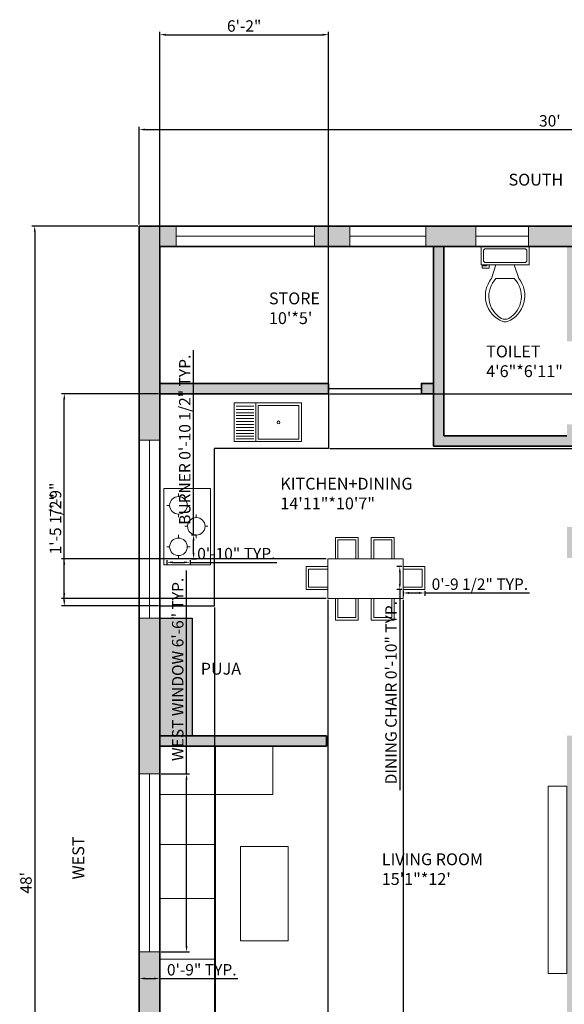
# Model space of a CAD drawing. Units: inches. Extents: x 2066 to 2563, y 1438 to 2142.
# Tile 2 of 3: x 2066 to 2304, y 1710 to 2142. Entities that reach past the tile are written whole.
import ezdxf

# ---------------------------------------------------------------- set-up
doc = ezdxf.new("R2010")
doc.units = ezdxf.units.IN
for name, color, linetype, lineweight in [('A-ANNO-DIMS', 2, 'Continuous', 18), ('A-ANNO-TEXT', 10, 'Continuous', 18), ('A-AREA-IDEN', 10, 'Continuous', 18), ('A-DOOR', 4, 'Continuous', 25), ('A-EQPM', 52, 'Continuous', 18), ('A-FLOR-CASE', 191, 'Continuous', 25), ('A-FLOR-CASE-PATT', 9, 'Continuous', 13), ('A-FLOR-FIXT', 8, 'Continuous', 18), ('A-WALL-PATT', 140, 'Continuous', 13), ('FUR', 191, 'Continuous', 18), ('KIT', 52, 'Continuous', 25), ('WALL', 7, 'Continuous', 35), ('WIND', 210, 'Continuous', 18)]:
    doc.layers.add(name, color=color, linetype=linetype, lineweight=lineweight)
doc.styles.get("Standard").update_dxf_attribs({"font": 'arial.ttf'})
doc.dimstyles.new('ISO-25', dxfattribs={"dimtxt": 5, "dimasz": 2.5, "dimexe": 1.25, "dimexo": 0.625, "dimtad": 1, "dimdec": 0, "dimlunit": 4, "dimtxsty": 'Standard', "dimcen": 2.5, "dimadec": 0, "dimazin": 0, "dimtfac": 1, "dimtdec": 0, "dimtmove": 0, "dimatfit": 3, "dimfxl": 1, "dimarcsym": 0})

# ---------------------------------------------------------------- blocks, each defined once
blk = doc.blocks.new('*U3')
for p, q in [((9.5, -6), (9.5, -2)), ((-10, -8.5), (-8, -8.5)), ((-10, -9.5), (-10, -8.5)), ((-8, -8.5), (-8, -8)), ((-7, -8), (-7, -9.5)), ((-4, -8), (-6, -14)), ((4, -8), (6, -14)), ((-7, -9.5), (-10, -9.5)), ((4, -14), (-4, -14))]:
    blk.add_line(p, q)
blk.add_lwpolyline([(10.5, -8), (10.5, 0), (-10.5, 0), (-10.5, -8)], close=True)
for points in [[(-9.5, -2), (-9.5, -6)], [(8.5, -1), (-8.5, -1)], [(-8.5, -7), (8.5, -7)]]:
    blk.add_lwpolyline(points)
for centre, radius, start, end in [((-8.62, -1.88), 0.884, 81.8699, 188.1301), ((8.62, -1.88), 0.884, 351.8699, 98.1301), ((-8.62, -6.12), 0.884, 171.8699, 278.1301), ((8.62, -6.12), 0.884, 261.8699, 8.1301), ((3.52, -21.58), 12.17, 141.4691, 247.9714), ((4.2, -21.82), 11.33, 136.3677, 238.9468), ((-3.52, -21.58), 12.17, 292.0284, 38.5307), ((-4.2, -21.82), 11.33, 301.053, 43.6321), ((0, -27.88), 4, 245.7318, 294.2682), ((0, -29), 4, 254.8605, 285.1395)]:
    blk.add_arc(centre, radius, start, end)
blk = doc.blocks.new('*D8')
at = {"layer": 'A-ANNO-DIMS', "color": 0, "lineweight": -2, "transparency": 16777216}
for p, q in [((2118.07, 2051.67), (2118.07, 2094.59)), ((2478.07, 2051.67), (2478.07, 2094.59)), ((2120.57, 2093.34), (2475.57, 2093.34))]:
    blk.add_line(p, q, dxfattribs=at)
at = {"layer": 'A-ANNO-DIMS', "color": 0, "lineweight": 100, "transparency": 16777216}
for points in [[(2120.57, 2093.76), (2120.57, 2092.93), (2118.07, 2093.34)], [(2475.57, 2093.76), (2475.57, 2092.93), (2478.07, 2093.34)]]:
    blk.add_solid(points, dxfattribs=at)
at = {"layer": 'Defpoints', "color": 0, "lineweight": 100, "transparency": 16777216}
for p in [(2478.07, 2093.34), (2118.07, 2051.04), (2478.07, 2051.04)]:
    blk.add_point(p, dxfattribs=at)
at = {"layer": 'A-ANNO-DIMS', "color": 0, "transparency": 16777216, "insert": (2298.07, 2096.52), "char_height": 5, "attachment_point": 5}
blk.add_mtext("30'", dxfattribs=at)
blk = doc.blocks.new('*D9')
at = {"layer": 'A-ANNO-DIMS', "color": 0, "lineweight": -2, "transparency": 16777216}
for p, q in [((2117.45, 2051.04), (2070.96, 2051.04)), ((2072.21, 2048.54), (2072.21, 1477.54)), ((2117.45, 1475.04), (2070.96, 1475.04))]:
    blk.add_line(p, q, dxfattribs=at)
at = {"layer": 'A-ANNO-DIMS', "color": 0, "lineweight": 100, "transparency": 16777216}
for points in [[(2071.79, 2048.54), (2072.63, 2048.54), (2072.21, 2051.04)], [(2071.79, 1477.54), (2072.63, 1477.54), (2072.21, 1475.04)]]:
    blk.add_solid(points, dxfattribs=at)
at = {"layer": 'Defpoints', "color": 0, "lineweight": 100, "transparency": 16777216}
for p in [(2118.07, 2051.04), (2072.21, 1475.04), (2118.07, 1475.04)]:
    blk.add_point(p, dxfattribs=at)
at = {"layer": 'A-ANNO-DIMS', "color": 0, "transparency": 16777216, "insert": (2069.03, 1763.04), "char_height": 5, "attachment_point": 5, "rotation": 90}
blk.add_mtext("48'", dxfattribs=at)
blk = doc.blocks.new('CHAIR-DINING')
for p, q in [((0, 0), (0, 9.41)), ((0, 9.41), (10.07, 9.41)), ((10.07, 9.41), (10.07, 0))]:
    blk.add_line(p, q)
blk.add_lwpolyline([(1.13, 0), (9, 0), (9, 8.36), (1.13, 8.36)], close=True)
blk = doc.blocks.new('COOKTOP-BURNER')
for p, q in [((5.08, 9.08), (5.08, 10.45)), ((0, 5.22), (1.22, 5.22)), ((8.93, 5.22), (10.15, 5.22)), ((5.08, 0), (5.08, 1.37))]:
    blk.add_line(p, q)
blk.add_circle((5.08, 5.22), 3.85)
blk = doc.blocks.new('WIN-78IN')
blk.add_line((4.5, 78.03), (4.5, 0))
blk.add_lwpolyline([(0, 0), (9, 0), (9, 78.03), (0, 78.03)], close=True)
blk = doc.blocks.new('*D16')
at = {"layer": 'A-ANNO-DIMS', "color": 0, "lineweight": -2, "transparency": 16777216}
for p, q in [((2233.18, 1901.72), (2231.04, 1901.72)), ((2232.29, 1899.22), (2232.29, 1894.15)), ((2233.18, 1891.65), (2231.04, 1891.65)), ((2232.29, 1891.65), (2232.29, 1803.73))]:
    blk.add_line(p, q, dxfattribs=at)
at = {"layer": 'A-ANNO-DIMS', "color": 0, "lineweight": 100, "transparency": 16777216}
for points in [[(2231.88, 1899.22), (2232.71, 1899.22), (2232.29, 1901.72)], [(2231.88, 1894.15), (2232.71, 1894.15), (2232.29, 1891.65)]]:
    blk.add_solid(points, dxfattribs=at)
at = {"layer": 'Defpoints', "color": 0, "lineweight": 100, "transparency": 16777216}
for p in [(2233.8, 1901.72), (2232.29, 1891.65), (2233.8, 1891.65)]:
    blk.add_point(p, dxfattribs=at)
at = {"layer": 'A-ANNO-DIMS', "color": 0, "transparency": 16777216, "insert": (2229.08, 1846.44), "char_height": 5, "attachment_point": 5, "rotation": 90}
blk.add_mtext('DINING CHAIR 0\'-10" TYP.', dxfattribs=at)
blk = doc.blocks.new('*D17')
at = {"layer": 'A-ANNO-DIMS', "color": 0, "lineweight": -2, "transparency": 16777216}
for p, q in [((2233.8, 1891.03), (2233.8, 1888.89)), ((2236.3, 1890.14), (2240.72, 1890.14)), ((2243.22, 1891.03), (2243.22, 1888.89)), ((2243.22, 1890.14), (2289.09, 1890.14))]:
    blk.add_line(p, q, dxfattribs=at)
at = {"layer": 'A-ANNO-DIMS', "color": 0, "lineweight": 100, "transparency": 16777216}
for points in [[(2236.3, 1890.56), (2236.3, 1889.72), (2233.8, 1890.14)], [(2240.72, 1890.56), (2240.72, 1889.72), (2243.22, 1890.14)]]:
    blk.add_solid(points, dxfattribs=at)
at = {"layer": 'Defpoints', "color": 0, "lineweight": 100, "transparency": 16777216}
for p in [(2233.8, 1891.65), (2243.22, 1891.65), (2243.22, 1890.14)]:
    blk.add_point(p, dxfattribs=at)
at = {"layer": 'A-ANNO-DIMS', "color": 0, "transparency": 16777216, "insert": (2267.4, 1893.35), "char_height": 5, "attachment_point": 5}
blk.add_mtext('0\'-9 1/2" TYP.', dxfattribs=at)
blk = doc.blocks.new('*D20')
at = {"layer": 'A-ANNO-DIMS', "color": 0, "lineweight": -2, "transparency": 16777216}
for p, q in [((2141.87, 1915.6), (2141.87, 1996.57)), ((2140.93, 1915.6), (2143.12, 1915.6)), ((2141.87, 1907.65), (2141.87, 1913.1)), ((2140.93, 1905.15), (2143.12, 1905.15))]:
    blk.add_line(p, q, dxfattribs=at)
at = {"layer": 'A-ANNO-DIMS', "color": 0, "lineweight": 100, "transparency": 16777216}
for points in [[(2141.45, 1913.1), (2142.29, 1913.1), (2141.87, 1915.6)], [(2141.45, 1907.65), (2142.29, 1907.65), (2141.87, 1905.15)]]:
    blk.add_solid(points, dxfattribs=at)
at = {"layer": 'Defpoints', "color": 0, "lineweight": 100, "transparency": 16777216}
for p in [(2140.3, 1915.6), (2141.87, 1915.6), (2140.3, 1905.15)]:
    blk.add_point(p, dxfattribs=at)
at = {"layer": 'A-ANNO-DIMS', "color": 0, "transparency": 16777216, "insert": (2138.66, 1957.34), "char_height": 5, "attachment_point": 5, "rotation": 90}
blk.add_mtext('BURNER 0\'-10 1/2" TYP.', dxfattribs=at)
blk = doc.blocks.new('*D21')
at = {"layer": 'A-ANNO-DIMS', "color": 0, "lineweight": -2, "transparency": 16777216}
for p, q in [((2130.15, 1904.52), (2130.15, 1902.33)), ((2140.3, 1904.52), (2140.3, 1902.33)), ((2132.65, 1903.58), (2137.8, 1903.58)), ((2140.3, 1903.58), (2178.41, 1903.58))]:
    blk.add_line(p, q, dxfattribs=at)
at = {"layer": 'A-ANNO-DIMS', "color": 0, "lineweight": 100, "transparency": 16777216}
for points in [[(2132.65, 1904), (2132.65, 1903.17), (2130.15, 1903.58)], [(2137.8, 1904), (2137.8, 1903.17), (2140.3, 1903.58)]]:
    blk.add_solid(points, dxfattribs=at)
at = {"layer": 'Defpoints', "color": 0, "lineweight": 100, "transparency": 16777216}
for p in [(2130.15, 1905.15), (2140.3, 1905.15), (2140.3, 1903.58)]:
    blk.add_point(p, dxfattribs=at)
at = {"layer": 'A-ANNO-DIMS', "color": 0, "transparency": 16777216, "insert": (2160.61, 1906.76), "char_height": 5, "attachment_point": 5}
blk.add_mtext('0\'-10" TYP.', dxfattribs=at)
blk = doc.blocks.new('*D24')
at = {"layer": 'A-ANNO-DIMS', "color": 0, "lineweight": -2, "transparency": 16777216}
for p, q in [((2138.78, 1810.83), (2138.78, 1899.97)), ((2127.7, 1810.83), (2140.03, 1810.83)), ((2138.78, 1735.3), (2138.78, 1808.33)), ((2127.7, 1732.8), (2140.03, 1732.8))]:
    blk.add_line(p, q, dxfattribs=at)
at = {"layer": 'A-ANNO-DIMS', "color": 0, "lineweight": 100, "transparency": 16777216}
for points in [[(2138.36, 1808.33), (2139.19, 1808.33), (2138.78, 1810.83)], [(2138.36, 1735.3), (2139.19, 1735.3), (2138.78, 1732.8)]]:
    blk.add_solid(points, dxfattribs=at)
at = {"layer": 'Defpoints', "color": 0, "lineweight": 100, "transparency": 16777216}
for p in [(2127.07, 1810.83), (2138.78, 1810.83), (2127.07, 1732.8)]:
    blk.add_point(p, dxfattribs=at)
at = {"layer": 'A-ANNO-DIMS', "color": 0, "transparency": 16777216, "insert": (2135.57, 1856.65), "char_height": 5, "attachment_point": 5, "rotation": 90}
blk.add_mtext('WEST WINDOW 6\'-6" TYP.', dxfattribs=at)
blk = doc.blocks.new('*D25')
at = {"layer": 'A-ANNO-DIMS', "color": 0, "lineweight": -2, "transparency": 16777216}
for p, q in [((2118.07, 1732.17), (2118.07, 1719.84)), ((2127.07, 1732.17), (2127.07, 1719.84)), ((2120.57, 1721.09), (2124.57, 1721.09)), ((2127.07, 1721.09), (2161.3, 1721.09))]:
    blk.add_line(p, q, dxfattribs=at)
at = {"layer": 'A-ANNO-DIMS', "color": 0, "lineweight": 100, "transparency": 16777216}
for points in [[(2120.57, 1721.51), (2120.57, 1720.68), (2118.07, 1721.09)], [(2124.57, 1721.51), (2124.57, 1720.68), (2127.07, 1721.09)]]:
    blk.add_solid(points, dxfattribs=at)
at = {"layer": 'Defpoints', "color": 0, "lineweight": 100, "transparency": 16777216}
for p in [(2118.07, 1732.8), (2127.07, 1732.8), (2127.07, 1721.09)]:
    blk.add_point(p, dxfattribs=at)
at = {"layer": 'A-ANNO-DIMS', "color": 0, "transparency": 16777216, "insert": (2145.44, 1724.27), "char_height": 5, "attachment_point": 5}
blk.add_mtext('0\'-9" TYP.', dxfattribs=at)
blk = doc.blocks.new('*D30')
at = {"layer": 'A-ANNO-DIMS', "color": 0, "lineweight": -2, "transparency": 16777216}
for p, q in [((2127.07, 1883.82), (2127.07, 1440.89)), ((2151.07, 1883.82), (2151.07, 1440.89)), ((2129.57, 1442.14), (2148.57, 1442.14))]:
    blk.add_line(p, q, dxfattribs=at)
at = {"layer": 'A-ANNO-DIMS', "color": 0, "lineweight": 100, "transparency": 16777216}
for points in [[(2129.57, 1442.56), (2129.57, 1441.73), (2127.07, 1442.14)], [(2148.57, 1442.56), (2148.57, 1441.73), (2151.07, 1442.14)]]:
    blk.add_solid(points, dxfattribs=at)
at = {"layer": 'Defpoints', "color": 0, "lineweight": 100, "transparency": 16777216}
for p in [(2127.07, 1884.45), (2151.07, 1884.45), (2151.07, 1442.14)]:
    blk.add_point(p, dxfattribs=at)
at = {"layer": 'A-ANNO-DIMS', "color": 0, "transparency": 16777216, "insert": (2139.07, 1445.32), "char_height": 5, "attachment_point": 5}
blk.add_mtext('2\'-0"', dxfattribs=at)
blk = doc.blocks.new('*D31')
at = {"layer": 'A-ANNO-DIMS', "color": 0, "lineweight": -2, "transparency": 16777216}
for p, q in [((2126.45, 1977.54), (2083.92, 1977.54)), ((2085.17, 1886.95), (2085.17, 1975.04)), ((2126.45, 1884.45), (2083.92, 1884.45))]:
    blk.add_line(p, q, dxfattribs=at)
at = {"layer": 'A-ANNO-DIMS', "color": 0, "lineweight": 100, "transparency": 16777216}
for points in [[(2084.76, 1975.04), (2085.59, 1975.04), (2085.17, 1977.54)], [(2084.76, 1886.95), (2085.59, 1886.95), (2085.17, 1884.45)]]:
    blk.add_solid(points, dxfattribs=at)
at = {"layer": 'Defpoints', "color": 0, "lineweight": 100, "transparency": 16777216}
for p in [(2085.17, 1977.54), (2127.07, 1977.54), (2127.07, 1884.45)]:
    blk.add_point(p, dxfattribs=at)
at = {"layer": 'A-ANNO-DIMS', "color": 0, "transparency": 16777216, "insert": (2082, 1931), "char_height": 5, "attachment_point": 5, "rotation": 90}
blk.add_mtext('7\'-9"', dxfattribs=at)
blk = doc.blocks.new('*D32')
at = {"layer": 'A-ANNO-DIMS', "color": 0, "lineweight": -2, "transparency": 16777216}
for p, q in [((2127.07, 1978.17), (2127.07, 2136.19)), ((2129.57, 2134.94), (2198.51, 2134.94)), ((2201.01, 1978.17), (2201.01, 2136.19))]:
    blk.add_line(p, q, dxfattribs=at)
at = {"layer": 'A-ANNO-DIMS', "color": 0, "lineweight": 100, "transparency": 16777216}
for points in [[(2129.57, 2135.36), (2129.57, 2134.53), (2127.07, 2134.94)], [(2198.51, 2135.36), (2198.51, 2134.53), (2201.01, 2134.94)]]:
    blk.add_solid(points, dxfattribs=at)
at = {"layer": 'Defpoints', "color": 0, "lineweight": 100, "transparency": 16777216}
for p in [(2201.01, 2134.94), (2127.07, 1977.54), (2201.01, 1977.54)]:
    blk.add_point(p, dxfattribs=at)
at = {"layer": 'A-ANNO-DIMS', "color": 0, "transparency": 16777216, "insert": (2164.04, 2138.12), "char_height": 5, "attachment_point": 5}
blk.add_mtext('6\'-2"', dxfattribs=at)
blk = doc.blocks.new('*D33')
at = {"layer": 'A-ANNO-DIMS', "color": 0, "lineweight": -2, "transparency": 16777216}
for p, q in [((2201.63, 1977.54), (2563.22, 1977.54)), ((2561.97, 1975.04), (2561.97, 1956.04)), ((2201.63, 1953.54), (2563.22, 1953.54))]:
    blk.add_line(p, q, dxfattribs=at)
at = {"layer": 'A-ANNO-DIMS', "color": 0, "lineweight": 100, "transparency": 16777216}
for points in [[(2561.56, 1975.04), (2562.39, 1975.04), (2561.97, 1977.54)], [(2561.56, 1956.04), (2562.39, 1956.04), (2561.97, 1953.54)]]:
    blk.add_solid(points, dxfattribs=at)
at = {"layer": 'Defpoints', "color": 0, "lineweight": 100, "transparency": 16777216}
for p in [(2201.01, 1977.54), (2201.01, 1953.54), (2561.97, 1953.54)]:
    blk.add_point(p, dxfattribs=at)
at = {"layer": 'A-ANNO-DIMS', "color": 0, "transparency": 16777216, "insert": (2558.8, 1965.54), "char_height": 5, "attachment_point": 5, "rotation": 90}
blk.add_mtext('2\'-0"', dxfattribs=at)
blk = doc.blocks.new('*D34')
at = {"layer": 'A-ANNO-DIMS', "color": 0, "lineweight": -2, "transparency": 16777216}
for p, q in [((2200.67, 1887.07), (2200.67, 1440.89)), ((2233.8, 1887.07), (2233.8, 1440.89)), ((2203.17, 1442.14), (2231.3, 1442.14))]:
    blk.add_line(p, q, dxfattribs=at)
at = {"layer": 'A-ANNO-DIMS', "color": 0, "lineweight": 100, "transparency": 16777216}
for points in [[(2203.17, 1442.56), (2203.17, 1441.73), (2200.67, 1442.14)], [(2231.3, 1442.56), (2231.3, 1441.73), (2233.8, 1442.14)]]:
    blk.add_solid(points, dxfattribs=at)
at = {"layer": 'Defpoints', "color": 0, "lineweight": 100, "transparency": 16777216}
for p in [(2200.67, 1887.69), (2233.8, 1887.69), (2233.8, 1442.14)]:
    blk.add_point(p, dxfattribs=at)
at = {"layer": 'A-ANNO-DIMS', "color": 0, "transparency": 16777216, "insert": (2217.24, 1445.32), "char_height": 5, "attachment_point": 5}
blk.add_mtext('2\'-9"', dxfattribs=at)
blk = doc.blocks.new('*D35')
at = {"layer": 'A-ANNO-DIMS', "color": 0, "lineweight": -2, "transparency": 16777216}
for p, q in [((2085.17, 1905.12), (2085.17, 1933.35)), ((2200.04, 1905.12), (2083.92, 1905.12)), ((2085.17, 1890.19), (2085.17, 1902.62)), ((2200.04, 1887.69), (2083.92, 1887.69))]:
    blk.add_line(p, q, dxfattribs=at)
at = {"layer": 'A-ANNO-DIMS', "color": 0, "lineweight": 100, "transparency": 16777216}
for points in [[(2084.76, 1902.62), (2085.59, 1902.62), (2085.17, 1905.12)], [(2084.76, 1890.19), (2085.59, 1890.19), (2085.17, 1887.69)]]:
    blk.add_solid(points, dxfattribs=at)
at = {"layer": 'Defpoints', "color": 0, "lineweight": 100, "transparency": 16777216}
for p in [(2085.17, 1905.12), (2200.67, 1905.12), (2200.67, 1887.69)]:
    blk.add_point(p, dxfattribs=at)
at = {"layer": 'A-ANNO-DIMS', "color": 0, "transparency": 16777216, "insert": (2081.96, 1920.48), "char_height": 5, "attachment_point": 5, "rotation": 90}
blk.add_mtext('1\'-5 1/2"', dxfattribs=at)

msp = doc.modelspace()

# ---------------------------------------------------------------- hatches: boundary and pattern name
at = {"layer": 'A-FLOR-CASE-PATT'}
h = msp.add_hatch(color=256, dxfattribs=at)
h.dxf.hatch_style = 1
h.paths.add_polyline_path([(2141.31, 1879.08), (2127.07, 1879.08), (2127.07, 1827.54), (2141.31, 1827.54)])
at = {"layer": 'A-WALL-PATT'}
h = msp.add_hatch(color=256, dxfattribs=at)
h.dxf.hatch_style = 1
h.paths.add_polyline_path([(2210.43, 2051.04), (2194.82, 2051.04), (2194.82, 2042.04), (2210.43, 2042.04)])
h.paths.add_polyline_path([(2265.69, 2051.04), (2243.73, 2051.04), (2243.73, 2042.04), (2265.69, 2042.04)])
h.paths.add_polyline_path([(2478.07, 2051.04), (2288.73, 2051.04), (2288.73, 2042.04), (2288.96, 2042.04), (2469.07, 2042.04), (2469.07, 2021.26), (2478.07, 2021.26)])
h.paths.add_polyline_path([(2127.07, 2042.04), (2134.17, 2042.04), (2134.17, 2051.04), (2118.07, 2051.04), (2118.07, 1957.11), (2127.07, 1957.11), (2127.07, 1977.54)])
h.paths.add_polyline_path([(2201.01, 1982.04), (2127.07, 1982.04), (2127.07, 1977.54), (2201.01, 1977.54)])
h.paths.add_polyline_path([(2247.07, 1982.04), (2241.78, 1982.04), (2241.78, 1977.54), (2247.07, 1977.54)])
h.paths.add_polyline_path([(2251.57, 2042.04), (2247.07, 2042.04), (2247.07, 1954.54), (2310.07, 1954.54), (2310.07, 1964.11), (2305.57, 1964.11), (2305.57, 1959.04), (2251.57, 1959.04)])
h.paths.add_polyline_path([(2310.07, 2042.04), (2305.57, 2042.04), (2305.57, 2000.54), (2310.07, 2000.54)], flags=17)
h.paths.add_polyline_path([(2478.07, 1938.37), (2469.07, 1938.37), (2469.07, 1846.24), (2478.07, 1846.24)])
h.paths.add_polyline_path([(2469.07, 1910.04), (2384.89, 1910.04), (2370.05, 1910.04), (2318.28, 1910.04), (2310.07, 1910.04), (2310.07, 1919.07), (2305.57, 1919.07), (2305.57, 1910.04), (2305.57, 1905.54), (2310.07, 1905.54), (2318.28, 1905.54), (2370.05, 1905.54), (2469.07, 1905.54)])
h.paths.add_polyline_path([(2469.07, 1868.54), (2408.15, 1868.54), (2408.15, 1858.69), (2412.15, 1858.69), (2412.15, 1864.54), (2469.07, 1864.54)])
h.paths.add_polyline_path([(2469.07, 1827.54), (2359.25, 1827.54), (2359.25, 1823.04), (2469.07, 1823.04)])
h.paths.add_polyline_path([(2314.44, 1827.54), (2310.07, 1827.54), (2305.57, 1827.54), (2305.57, 1743.86), (2305.57, 1723.24), (2305.57, 1679.04), (2305.57, 1674.54), (2322.38, 1674.54), (2380.79, 1674.54), (2397.77, 1674.54), (2415.18, 1674.54), (2415.18, 1679.04), (2310.07, 1679.04), (2310.07, 1823.04), (2314.44, 1823.04)])
h.paths.add_polyline_path([(2478.07, 1763.36), (2469.07, 1763.36), (2469.07, 1655.36), (2478.07, 1655.36)])
h.paths.add_polyline_path([(2469.07, 1679.04), (2446.03, 1679.04), (2446.03, 1674.54), (2469.07, 1674.54)])
h.paths.add_polyline_path([(2410.07, 1670.54), (2410.07, 1674.54), (2405.57, 1674.54), (2405.57, 1670.54), (2405.57, 1590.09), (2410.07, 1590.09), (2410.07, 1593.54)])
h.paths.add_polyline_path([(2469.07, 1598.04), (2410.07, 1598.04), (2410.07, 1593.54), (2469.07, 1593.54)])
h.paths.add_polyline_path([(2478.07, 1622.1), (2469.07, 1622.1), (2469.07, 1578.59), (2478.07, 1578.59)])
h.paths.add_polyline_path([(2478.07, 1545.33), (2469.07, 1545.33), (2469.07, 1521.54), (2384.6, 1521.54), (2384.6, 1512.54), (2473.57, 1512.54), (2478.07, 1512.54)])
h.paths.add_polyline_path([(2410.07, 1558.62), (2405.57, 1558.62), (2405.57, 1521.54), (2410.07, 1521.54)])
h.paths.add_polyline_path([(2478.07, 1512.54), (2473.57, 1512.54), (2473.57, 1479.54), (2263.07, 1479.54), (2251.16, 1479.54), (2251.16, 1475.04), (2478.07, 1475.04)])
h.paths.add_polyline_path([(2122.57, 1674.54), (2118.07, 1674.54), (2118.07, 1475.04), (2131.87, 1475.04), (2131.87, 1479.54), (2122.57, 1479.54)])
h.paths.add_polyline_path([(2267.57, 1674.54), (2263.07, 1674.54), (2263.07, 1521.54), (2267.57, 1521.54)])
h.paths.add_polyline_path([(2270.46, 1679.04), (2259.18, 1679.04), (2259.18, 1674.54), (2263.07, 1674.54), (2270.46, 1674.54)])
h.paths.add_polyline_path([(2198.77, 1679.04), (2190.12, 1679.04), (2190.12, 1674.54), (2198.77, 1674.54)])
h.paths.add_polyline_path([(2139.93, 1679.04), (2127.07, 1679.04), (2127.07, 1674.54), (2139.93, 1674.54)])
h.paths.add_polyline_path([(2127.07, 1700.37), (2127.07, 1732.8), (2118.07, 1732.8), (2118.07, 1674.54), (2122.57, 1674.54), (2127.07, 1674.54), (2127.07, 1679.04)])
h.paths.add_polyline_path([(2127.07, 1879.08), (2118.07, 1879.08), (2118.07, 1810.83), (2127.07, 1810.83), (2127.07, 1823.04)])
h.paths.add_polyline_path([(2200.14, 1827.54), (2127.07, 1827.54), (2127.07, 1823.04), (2151.5, 1823.04), (2176.6, 1823.04), (2200.14, 1823.04)])

# ---------------------------------------------------------------- linework, layer by layer
at = {"layer": 'A-DOOR'}
msp.add_line((2201.01, 1979.79), (2241.78, 1979.79), dxfattribs=at)
at = {"layer": 'A-EQPM'}
msp.add_lwpolyline([(2128.79, 1902.53), (2149.34, 1902.53), (2149.34, 1935.94), (2128.79, 1935.94)], close=True, dxfattribs=at)
at = {"layer": 'A-FLOR-CASE'}
msp.add_lwpolyline([(2127.07, 1879.08), (2141.31, 1879.08), (2141.31, 1827.54), (2127.07, 1827.54)], close=True, dxfattribs=at)
at = {"layer": 'A-FLOR-FIXT'}
for p, q in [((2169.21, 1973.45), (2169.21, 1956.59)), ((2160.49, 1972.01), (2168.31, 1972.01)), ((2160.49, 1970.66), (2168.31, 1970.66)), ((2160.49, 1969.2), (2168.31, 1969.2)), ((2160.49, 1967.9), (2168.31, 1967.9)), ((2160.49, 1966.6), (2168.31, 1966.6)), ((2160.49, 1965.4), (2168.31, 1965.4)), ((2160.49, 1964), (2168.31, 1964)), ((2160.49, 1962.74), (2168.31, 1962.74)), ((2160.49, 1961.39), (2168.31, 1961.39)), ((2160.49, 1960.14), (2168.31, 1960.14)), ((2160.49, 1958.89), (2168.31, 1958.89)), ((2160.49, 1957.79), (2168.31, 1957.79))]:
    msp.add_line(p, q, dxfattribs=at)
for points in [[(2159.71, 1973.45), (2189.13, 1973.45), (2189.13, 1956.59), (2159.71, 1956.59)], [(2170.26, 1972.31), (2187.96, 1972.31), (2187.96, 1957.58), (2170.26, 1957.58)]]:
    msp.add_lwpolyline(points, close=True, dxfattribs=at)
msp.add_circle((2179.11, 1964.95), 0.627, dxfattribs=at)
at = {"layer": 'FUR'}
for p, q in [((2127.07, 1779.89), (2151.5, 1779.89)), ((2127.07, 1756.23), (2151.5, 1756.23)), ((2127.07, 1729.54), (2151.5, 1729.54))]:
    msp.add_line(p, q, dxfattribs=at)
for points in [[(2200.67, 1905.12), (2233.8, 1905.12), (2233.8, 1887.69), (2200.67, 1887.69)], [(2176.6, 1823.04), (2127.07, 1823.04), (2127.07, 1801.72), (2176.6, 1801.72)], [(2127.07, 1823.04), (2151.5, 1823.04), (2151.5, 1679.04), (2127.07, 1679.04)], [(2305.57, 1805.39), (2297.27, 1805.39), (2297.27, 1723.24), (2305.57, 1723.24)], [(2162.42, 1737.61), (2183.37, 1737.61), (2183.37, 1779.02), (2162.42, 1779.02)]]:
    msp.add_lwpolyline(points, close=True, dxfattribs=at)
at = {"layer": 'KIT'}
for p, q in [((2201.01, 1977.54), (2201.01, 1953.54)), ((2201.01, 1953.54), (2151, 1953.54)), ((2151.07, 1884.45), (2151.07, 1953.54)), ((2127.07, 1884.45), (2151.07, 1884.45))]:
    msp.add_line(p, q, dxfattribs=at)
at = {"layer": 'WALL'}
for p, q in [((2118.07, 2051.04), (2478.07, 2051.04)), ((2118.07, 1475.04), (2118.07, 2051.04)), ((2127.07, 2042.04), (2469.07, 2042.04)), ((2127.07, 2042.04), (2247.07, 2042.04)), ((2127.07, 1674.54), (2127.07, 2042.04)), ((2247.07, 2042.04), (2247.07, 1982.04)), ((2247.07, 2042.04), (2247.07, 1954.54)), ((2251.57, 2042.04), (2251.57, 1977.54)), ((2251.57, 2042.04), (2251.57, 1959.04)), ((2201.01, 1982.04), (2127.07, 1982.04)), ((2201.01, 1982.04), (2201.01, 1977.54)), ((2247.07, 1982.04), (2241.78, 1982.04)), ((2127.07, 1977.54), (2127.07, 1827.54)), ((2201.01, 1977.54), (2127.07, 1977.54)), ((2247.07, 1977.54), (2241.78, 1977.54)), ((2251.57, 1959.04), (2305.57, 1959.04)), ((2247.07, 1954.54), (2310.07, 1954.54)), ((2127.07, 1827.54), (2200.14, 1827.54)), ((2200.14, 1827.54), (2200.14, 1823.04)), ((2127.07, 1823.04), (2200.14, 1823.04)), ((2127.07, 1823.04), (2127.07, 1679.04))]:
    msp.add_line(p, q, dxfattribs=at)
msp.add_lwpolyline([(2241.78, 1982.04), (2241.78, 1982.04), (2241.78, 1977.54), (2241.78, 1977.54)], close=True, dxfattribs=at)
at = {"layer": 'WIND'}
for p, q in [((2134.17, 2046.54), (2194.82, 2046.54)), ((2210.43, 2046.54), (2243.73, 2046.54)), ((2265.69, 2046.54), (2288.73, 2046.54))]:
    msp.add_line(p, q, dxfattribs=at)
for points in [[(2134.17, 2051.04), (2194.82, 2051.04), (2194.82, 2042.04), (2134.17, 2042.04)], [(2243.73, 2042.04), (2210.43, 2042.04), (2210.43, 2051.04), (2243.73, 2051.04)], [(2265.69, 2042.04), (2288.73, 2042.04), (2288.73, 2051.04), (2265.69, 2051.04)]]:
    msp.add_lwpolyline(points, close=True, dxfattribs=at)

# ---------------------------------------------------------------- block references
at = {"layer": 'A-EQPM'}
for p in [(2130.15, 1923.35), (2137.97, 1914.15), (2130.15, 1905.15)]:
    msp.add_blockref('COOKTOP-BURNER', p, dxfattribs=at)
at = {"layer": 'A-FLOR-FIXT'}
msp.add_blockref('*U3', (2278.46, 2042.04), dxfattribs=at)
at = {"layer": 'FUR'}
for p in [(2204.03, 1905.12), (2219.73, 1905.12)]:
    msp.add_blockref('CHAIR-DINING', p, dxfattribs=at)
at = {"layer": 'FUR', "extrusion": (0, 0, -1), "zscale": -1}
for p, rotation in [((-2200.67, 1901.72), 269.9999999999988), ((-2204.03, 1887.69), 180), ((-2219.73, 1887.69), 180)]:
    msp.add_blockref('CHAIR-DINING', p, dxfattribs=dict(at, rotation=rotation))
at = {"layer": 'FUR', "rotation": 269.9999999999988}
msp.add_blockref('CHAIR-DINING', (2233.8, 1901.72), dxfattribs=at)
at = {"layer": 'WIND'}
for p in [(2118.07, 1879.08), (2118.07, 1732.8)]:
    msp.add_blockref('WIN-78IN', p, dxfattribs=at)

# ---------------------------------------------------------------- texts
at = {"layer": 'A-ANNO-TEXT', "insert": (2279.98, 2073.97), "char_height": 5.193, "attachment_point": 1}
msp.add_mtext_dynamic_manual_height_columns('SOUTH', width=129.7814, gutter_width=25.96, heights=[0], dxfattribs=at)
at = {"layer": 'A-ANNO-TEXT', "insert": (2088.72, 1764.51), "char_height": 5.193, "attachment_point": 1, "rotation": 90}
msp.add_mtext_dynamic_manual_height_columns('WEST', width=129.7814, gutter_width=25.96, heights=[0], dxfattribs=at)
at = {"layer": 'A-AREA-IDEN', "attachment_point": 1}
for s, insert, char_height in [("STORE\\P10'*5'", (2174.91, 2021.91), 5.193), ('TOILET\\P4\'6"*6\'11"', (2270.17, 1998.65), 5.193), ('KITCHEN+DINING\\P14\'11"*10\'7"', (2179.92, 1940.66), 5.1929), ('PUJA', (2145, 1859.52), 5.193), ('LIVING ROOM\\P15\'1"*12\'', (2224.38, 1775.97), 5.1929)]:
    msp.add_mtext_dynamic_manual_height_columns(s, width=129.7814, gutter_width=25.96, heights=[0], dxfattribs=dict(at, insert=insert, char_height=char_height))

# ---------------------------------------------------------------- dimensions: what is measured, and where the dimension line sits
at = {"layer": 'A-ANNO-DIMS'}
for base, p1, p2, override, picture, middle in [((2201.01, 2134.94), (2127.07, 1977.54), (2201.01, 1977.54), {"dimdec": 1, "dimlfac": 1, "dimrnd": 0, "dimzin": 1, "dimdsep": 46, "dimlunit": 4, "dimfrac": 2}, '*D32', (2164.04, 2138.12)), ((2478.07, 2093.34), (2118.07, 2051.04), (2478.07, 2051.04), {"dimclrd": 0, "dimclre": 0, "dimclrt": 0}, '*D8', (2298.07, 2096.52)), ((2233.8, 1442.14), (2200.67, 1887.69), (2233.8, 1887.69), {"dimdec": 1, "dimlfac": 1, "dimrnd": 0, "dimzin": 1, "dimdsep": 46, "dimlunit": 4, "dimfrac": 2}, '*D34', (2217.24, 1445.32)), ((2151.07, 1442.14), (2127.07, 1884.45), (2151.07, 1884.45), {"dimdec": 1, "dimlfac": 1, "dimrnd": 0, "dimzin": 1, "dimdsep": 46, "dimlunit": 4, "dimfrac": 2}, '*D30', (2139.07, 1445.32))]:
    dim = msp.add_linear_dim(base=base, p1=p1, p2=p2, dimstyle='ISO-25', override=override, dxfattribs=at)
    dim.commit()
    dim.dimension.update_dxf_attribs({"geometry": picture, "text_midpoint": middle})
for base, p1, p2, override, picture, middle in [((2072.21, 1475.04), (2118.07, 2051.04), (2118.07, 1475.04), {"dimclrd": 0, "dimclre": 0, "dimclrt": 0}, '*D9', (2069.03, 1763.04)), ((2085.17, 1977.54), (2127.07, 1884.45), (2127.07, 1977.54), {"dimdec": 1, "dimlfac": 1, "dimrnd": 0, "dimzin": 1, "dimdsep": 46, "dimlunit": 4, "dimfrac": 2}, '*D31', (2082, 1931)), ((2561.97, 1953.54), (2201.01, 1977.54), (2201.01, 1953.54), {"dimdec": 1, "dimlfac": 1, "dimrnd": 0, "dimzin": 1, "dimdsep": 46, "dimlunit": 4, "dimfrac": 2}, '*D33', (2558.8, 1965.54)), ((2085.17, 1905.12), (2200.67, 1887.69), (2200.67, 1905.12), {"dimdec": 1, "dimlfac": 1, "dimrnd": 0, "dimzin": 1, "dimdsep": 46, "dimlunit": 4, "dimfrac": 2}, '*D35', (2081.96, 1920.48))]:
    dim = msp.add_linear_dim(base=base, p1=p1, p2=p2, angle=90, dimstyle='ISO-25', override=override, dxfattribs=at)
    dim.commit()
    dim.dimension.update_dxf_attribs({"geometry": picture, "text_midpoint": middle})
for base, p1, p2, angle, text, picture, middle in [((2141.8694, 1915.5966), (2140.3024, 1905.1499), (2140.3024, 1915.5966), 90, 'BURNER <> TYP.', '*D20', (2138.6591, 1957.3352)), ((2138.78, 1810.83), (2127.07, 1732.8), (2127.07, 1810.83), 90, 'WEST WINDOW <> TYP.', '*D24', (2135.57, 1856.65)), ((2232.29, 1891.65), (2233.8, 1901.72), (2233.8, 1891.65), 270, 'DINING CHAIR <> TYP.', '*D16', (2229.08, 1846.44))]:
    dim = msp.add_linear_dim(base=base, p1=p1, p2=p2, angle=angle, text=text, dimstyle='ISO-25', override={"dimdec": 1, "dimlfac": 1, "dimrnd": 0, "dimzin": 1, "dimdsep": 46, "dimlunit": 4, "dimfrac": 2}, dxfattribs=at)
    dim.commit()
    dim.dimension.update_dxf_attribs({"geometry": picture, "text_midpoint": middle})
for base, p1, p2, picture, middle in [((2140.3024, 1903.5829), (2130.1511, 1905.1499), (2140.3024, 1905.1499), '*D21', (2160.6085, 1906.7607)), ((2243.22, 1890.14), (2233.8, 1891.65), (2243.22, 1891.65), '*D17', (2267.4, 1893.35)), ((2127.07, 1721.09), (2118.07, 1732.8), (2127.07, 1732.8), '*D25', (2145.44, 1724.27))]:
    dim = msp.add_linear_dim(base=base, p1=p1, p2=p2, text='<> TYP.', dimstyle='ISO-25', override={"dimdec": 1, "dimlfac": 1, "dimrnd": 0, "dimzin": 1, "dimdsep": 46, "dimlunit": 4, "dimfrac": 2}, dxfattribs=at)
    dim.commit()
    dim.dimension.update_dxf_attribs({"geometry": picture, "text_midpoint": middle})

doc.saveas('drawing.dxf')
